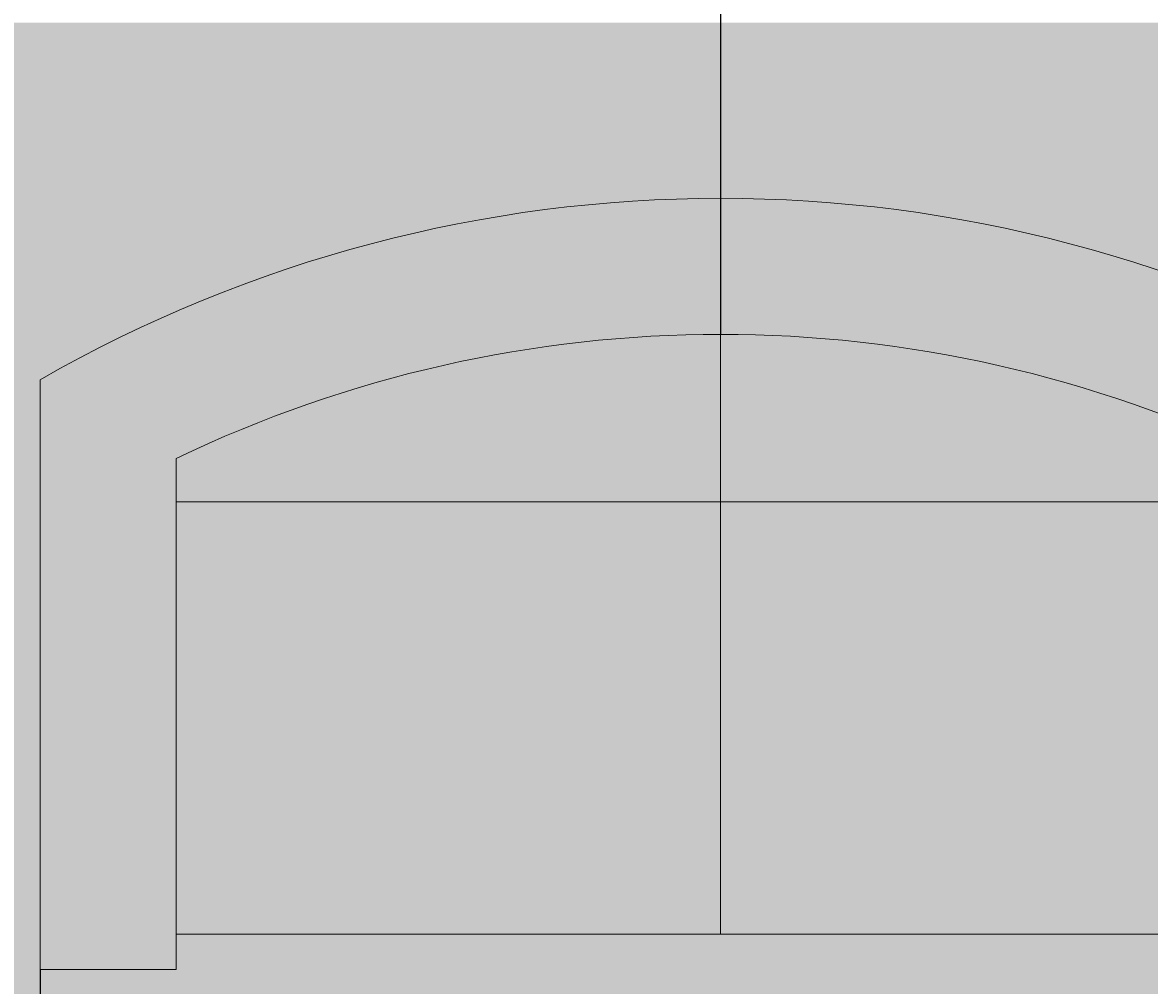
# Model space of a CAD drawing. Units: millimetres. Extents: x -229 to 16545, y -10488 to 4272.
# Tile 21 of 29: x 11572 to 12629, y -2111 to -1208. Entities that reach past the tile are written whole.
import ezdxf

# ---------------------------------------------------------------- set-up
doc = ezdxf.new("R2010")
doc.units = ezdxf.units.MM
for name, color, linetype, lineweight in [('A-ANNO-DIMS', 2, 'Continuous', 18), ('A-FURN', 8, 'Continuous', 18), ('A-FURN-PATT', 252, 'Continuous', 13)]:
    doc.layers.add(name, color=color, linetype=linetype, lineweight=lineweight)
doc.layers.add('A-FLOR-PATT', color=254, linetype='Continuous', lineweight=13, true_color=0xfeeab9)
doc.styles.get("Standard").update_dxf_attribs({"font": 'arial.ttf'})
doc.dimstyles.get("Standard").update_dxf_attribs({"dimtxt": 0.18, "dimasz": 0.18, "dimexe": 0.18, "dimexo": 0.0625, "dimgap": 0.09, "dimtad": 0, "dimtih": 1, "dimtoh": 1, "dimdec": 4, "dimzin": 0, "dimdsep": 46, "dimtxsty": 'Standard', "dimcen": 0.09, "dimadec": 0, "dimazin": 0, "dimtfac": 1, "dimtdec": 4, "dimtofl": 0, "dimtmove": 0, "dimatfit": 3, "dimfxl": 1, "dimtolj": 1, "dimtzin": 0, "dimarcsym": 0})

# ---------------------------------------------------------------- blocks, each defined once
blk = doc.blocks.new('Sofa - Roundback Loveseat 5 ft.')
for p, q in [((0, -32.44198), (0, -5.99998)), ((-24, -33.99998), (-24, -11.46958)), ((-23.9998, -13.38178), (23.99986, -13.38178)), ((-24, -32.44198), (24.00004, -32.44198))]:
    blk.add_line(p, q)
blk.add_lwpolyline([(-24, -33.99998), (-30, -33.99998), (-30, -7.99998)])
for centre, radius, start, end in [((0, -60.24998), 60.24998, 60.13715, 119.8628), ((0, -61.38438), 55.38444, 64.32083, 115.6792)]:
    blk.add_arc(centre, radius, start, end)
blk = doc.blocks.new('*D39')
at = {"layer": 'A-ANNO-DIMS', "color": 0, "lineweight": -2, "transparency": 16777216}
for p, q in [((11588.8, -2096.3), (11588.8, -2287.9)), ((12864.9, -2096.3), (12864.9, -2287.9)), ((11588.9, -2287.7), (12225.8, -2287.7)), ((12864.7, -2287.7), (12227.9, -2287.7))]:
    blk.add_line(p, q, dxfattribs=at)
at = {"layer": 'A-ANNO-DIMS', "color": 0, "transparency": 16777216}
for points in [[(11588.9, -2287.7), (11588.9, -2287.7), (11588.8, -2287.7)], [(12864.7, -2287.7), (12864.7, -2287.7), (12864.9, -2287.7)]]:
    blk.add_solid(points, dxfattribs=at)
at = {"layer": 'Defpoints', "color": 0, "transparency": 16777216}
for p in [(11588.8, -2096.3), (12864.9, -2096.3), (12864.9, -2287.7)]:
    blk.add_point(p, dxfattribs=at)
at = {"layer": 'A-ANNO-DIMS', "color": 0, "transparency": 16777216, "insert": (12226.8, -2287.7), "char_height": 0.18, "attachment_point": 5}
blk.add_mtext('\\A1;LOVESEAT 1276', dxfattribs=at)
blk = doc.blocks.new('*D103')
at = {"layer": 'A-ANNO-DIMS', "color": 0, "lineweight": -2, "transparency": 16777216}
for p, q in [((12227, -604.2), (12226.8, -604.2)), ((12226.8, -604.2), (12226.8, -1372.9)), ((12226.7, -2654.6), (12226.9, -2654.6)), ((12226.8, -2654.7), (12226.8, -2654.5))]:
    blk.add_line(p, q, dxfattribs=at)
at = {"layer": 'A-ANNO-DIMS', "color": 0, "transparency": 16777216}
blk.add_solid([(12226.8, -1372.9), (12226.9, -1372.9), (12226.8, -1373.1)], dxfattribs=at)
at = {"layer": 'Defpoints', "color": 0, "transparency": 16777216}
for p in [(12226.8, -1373.1), (12226.8, -2654.6)]:
    blk.add_point(p, dxfattribs=at)
at = {"layer": 'A-ANNO-DIMS', "color": 0, "transparency": 16777216, "insert": (12227.6, -604.2), "char_height": 0.18, "attachment_point": 5}
blk.add_mtext('\\A1;R1281.5', dxfattribs=at)
blk = doc.blocks.new('*D104')
at = {"layer": 'A-ANNO-DIMS', "color": 0, "lineweight": -2, "transparency": 16777216}
for p, q in [((12227, -793.9), (12226.8, -793.9)), ((12226.8, -793.9), (12226.8, -1500.5)), ((12226.7, -2678.7), (12226.9, -2678.7)), ((12226.8, -2678.8), (12226.8, -2678.6))]:
    blk.add_line(p, q, dxfattribs=at)
at = {"layer": 'A-ANNO-DIMS', "color": 0, "transparency": 16777216}
blk.add_solid([(12226.8, -1500.5), (12226.9, -1500.5), (12226.8, -1500.7)], dxfattribs=at)
at = {"layer": 'Defpoints', "color": 0, "transparency": 16777216}
for p in [(12226.8, -1500.7), (12226.8, -2678.7)]:
    blk.add_point(p, dxfattribs=at)
at = {"layer": 'A-ANNO-DIMS', "color": 0, "transparency": 16777216, "insert": (12227.5, -793.9), "char_height": 0.18, "attachment_point": 5}
blk.add_mtext('\\A1;R1178', dxfattribs=at)

msp = doc.modelspace()

# ---------------------------------------------------------------- hatches: boundary and pattern name
at = {"layer": 'A-FLOR-PATT', "transparency": 33554592}
h = msp.add_hatch(color=256, dxfattribs=at)
h.dxf.hatch_style = 1
h.paths.add_polyline_path([(7975.933, -5325.772), (7943.121, -5325.772), (7943.121, -4576.49, 0.40145271), (7225.933, -5325.772, 0.40145271), (6508.746, -4576.49), (6508.746, -5325.772), (6475.933, -5325.772), (6475.933, -5438.272), (5975.933, -5438.272), (5975.933, -7267.724), (5975.933, -7438.272), (6478.619, -7438.272), (6463.448, -7355.919), (6464.88, -7356.837), (6463.849, -7358.097), (6478.619, -7438.272), (6610.327, -7438.272), (6632.656, -7409.564), (6632.525, -7406.967), (6634.208, -7407.569), (6619.273, -7426.77), (6654.466, -7438.272), (7610.517, -7438.272), (7607.41, -7421.409), (7608.842, -7422.327), (7607.812, -7423.587), (7610.517, -7438.272), (7975.933, -7438.272)])
h.paths.add_polyline_path([(13785.933, -1208.272), (9555.933, -1208.272), (9555.933, -961.785), (9705.933, -961.785), (9705.933, -918.035), (10704.976, -918.035, 0.40145271), (9705.933, 38.215), (9555.933, 38.215), (9555.933, 2021.728), (5975.933, 2021.728), (5975.933, 755.492), (5745.933, 755.492), (5745.933, 1427.266), (2918.813, 1427.266), (2918.813, -492.942), (5013.319, -492.942), (5013.319, -978.272), (5745.933, -978.272), (5745.933, -397.513), (5975.933, -397.513), (5975.933, -1208.272), (4560.933, -1208.272), (4560.933, -1265.772), (4448.433, -1265.772), (4448.433, -1298.585), (4445.933, -1298.585), (3699.151, -1298.585, 0.40145271), (4448.433, -2015.772), (4560.933, -2015.772), (4560.933, -2384.177), (5745.933, -2384.177), (5799.402, -2384.177), (5799.402, -4518.272), (5975.933, -4518.272), (5975.933, -5208.272), (6475.933, -5208.272), (6475.933, -4575.772), (6508.746, -4575.772), (6508.746, -4576.49, -0.35647263), (7216.672, -5208.272), (7235.194, -5208.272, -0.35647263), (7943.121, -4576.49), (7943.121, -4575.772), (7975.933, -4575.772), (7975.933, -5208.272), (11176.247, -5208.272), (11159.44, -5191.465), (10520.768, -5191.465), (10520.768, -4888.936), (10571.19, -4888.936), (10571.19, -4872.129), (10772.876, -4872.129), (10772.876, -4888.936), (10789.683, -4888.936), (10789.683, -4872.129), (10991.368, -4872.129), (10991.368, -4888.936), (11041.79, -4888.936), (11041.79, -4872.129), (11058.597, -4872.129, -0.09090909), (11428.354, -4872.129), (11445.162, -4872.129), (11445.162, -4888.936), (11529.197, -4888.936), (11529.197, -5191.465), (11327.512, -5191.465), (11310.704, -5208.272), (13785.933, -5208.272)])
h.paths.add_polyline_path([(11047.216, -1630.944, -1), (11402.816, -1630.944, -1)], flags=16)
h.paths.add_polyline_path([(11148.816, -1630.944), (11225.016, -1554.744), (11301.216, -1630.944), (11225.016, -1707.144)], flags=0)
h.paths.add_polyline_path([(11199.616, -1630.944, -1), (11250.416, -1630.944, -1)], flags=0)
h.paths.add_polyline_path([(11588.751, -2096.259), (11588.751, -1543.254, -0.26666697), (12864.918, -1543.254), (12864.918, -2096.259), (12737.302, -2096.259), (12737.302, -2063.121), (11716.368, -2063.121), (11716.368, -2096.259)], flags=16)
h.paths.add_polyline_path([(12012.696, -2489.42), (12600.997, -2489.42), (12600.997, -3666.022), (12012.696, -3666.022)], flags=16)
h.paths.add_polyline_path([(12176.41, -3599.403), (12174.938, -3609.076), (12173.789, -3618.819), (12173.09, -3628.559), (12172.973, -3638.221), (12173.89, -3652.852), (12175.008, -3657.025), (12172.909, -3643.473), (12173.142, -3624.297), (12175.386, -3605.273)], flags=0)
h.paths.add_polyline_path([(8026.289, -286.944), (7737.703, -287.19), (7734.87, -269.156), (8029.092, -268.905)], flags=16)
h.paths.add_polyline_path([(7733.453, -260.139), (7710.784, -115.865), (7557.191, -115.996), (7556.999, 109.744), (7412.687, 132.166), (7412.433, 429.206), (7556.707, 451.876), (7556.568, 614.769), (7412.256, 637.19), (7412.003, 934.231), (7556.276, 956.9), (7556.084, 1182.639), (7709.677, 1182.77), (7732.099, 1327.082), (8029.14, 1327.335), (8051.808, 1183.062), (8205.401, 1183.192), (8205.594, 957.454), (8349.906, 935.031), (8350.159, 637.99), (8205.885, 615.322), (8206.024, 452.43), (8350.336, 430.006), (8350.59, 132.965), (8206.316, 110.298), (8206.509, -115.442), (8052.916, -115.573), (8030.493, -259.885)], flags=16)
h.paths.add_polyline_path([(12261.416, -3475.554), (12262.632, -3486.776), (12264.032, -3497.007), (12265.554, -3506.365), (12267.136, -3514.968), (12268.719, -3522.935), (12271.304, -3535.59), (12273.606, -3548.078), (12275.271, -3561.064), (12275.93, -3574.938), (12275.325, -3590.3), (12273.425, -3607.964), (12270.795, -3625.658), (12268.066, -3641.063), (12266.318, -3649.679), (12265.456, -3653.626), (12263.984, -3659.846), (12264.032, -3659.566), (12264.342, -3658.241), (12264.807, -3656.37), (12265.456, -3653.626), (12266.318, -3649.679), (12267.409, -3644.302), (12268.668, -3637.664), (12270.019, -3630.037), (12271.384, -3621.695), (12272.69, -3612.908), (12273.857, -3603.948), (12274.81, -3595.088), (12275.47, -3586.601), (12275.782, -3578.689), (12275.757, -3571.292), (12275.423, -3564.275), (12274.816, -3557.512), (12273.964, -3550.872), (12272.896, -3544.224), (12271.645, -3537.439), (12270.24, -3530.385), (12267.543, -3517.181), (12264.612, -3501.247), (12261.849, -3481.059)], flags=0)
h.paths.add_polyline_path([(12332.136, -3408.03), (12333.483, -3416.79), (12335.077, -3424.54), (12336.915, -3431.355), (12338.991, -3437.32), (12341.266, -3442.55), (12343.694, -3447.166), (12346.229, -3451.292), (12348.826, -3455.051), (12351.438, -3458.563), (12357.476, -3466.491), (12363.61, -3476.575), (12368.309, -3489.762), (12369.929, -3503.427), (12369.842, -3516.511), (12368.43, -3530.867), (12365.816, -3545.835), (12362.382, -3559.786), (12360.968, -3564.487), (12363.063, -3557.021), (12364.898, -3549.566), (12366.473, -3542.077), (12367.773, -3534.631), (12368.781, -3527.301), (12369.483, -3520.162), (12369.863, -3513.291), (12369.906, -3506.759), (12369.599, -3500.643), (12368.93, -3494.999), (12367.924, -3489.796), (12366.61, -3484.994), (12365.024, -3480.542), (12363.19, -3476.399), (12361.141, -3472.516), (12358.909, -3468.847), (12356.525, -3465.347), (12354.02, -3461.954), (12351.438, -3458.563), (12345.462, -3450.529), (12339.923, -3439.996), (12335.85, -3428.296), (12332.68, -3412.888)], flags=0)
h.paths.add_polyline_path([(12385.287, -3334.612), (12384.977, -3342.409), (12385.02, -3349.196), (12385.4, -3355.066), (12386.104, -3360.105), (12387.112, -3364.41), (12388.412, -3368.071), (12389.987, -3371.181), (12391.823, -3373.832), (12393.919, -3376.097), (12396.337, -3377.978), (12399.153, -3379.462), (12402.445, -3380.531), (12406.289, -3381.172), (12410.758, -3381.371), (12415.935, -3381.106), (12421.893, -3380.368), (12428.658, -3379.159), (12436.069, -3377.55), (12443.907, -3375.635), (12451.961, -3373.505), (12460.015, -3371.254), (12467.853, -3368.971), (12475.263, -3366.749), (12482.029, -3364.68), (12491.877, -3361.657), (12497.701, -3360.107), (12501.639, -3359.288), (12510.135, -3358.326), (12519.662, -3365.412), (12524.243, -3378.911), (12523.764, -3390.7), (12520.746, -3401.577), (12514.248, -3415.634), (12511.518, -3420.418), (12515.856, -3412.154), (12519.153, -3405.024), (12521.516, -3398.804), (12523.049, -3393.276), (12523.865, -3388.212), (12524.059, -3383.441), (12523.7, -3378.958), (12522.853, -3374.815), (12521.576, -3371.054), (12519.931, -3367.722), (12517.982, -3364.865), (12515.786, -3362.529), (12513.405, -3360.758), (12510.877, -3359.588), (12508.136, -3358.982), (12505.086, -3358.897), (12501.639, -3359.288), (12497.701, -3360.107), (12493.183, -3361.309), (12487.988, -3362.851), (12476.403, -3366.408), (12463.335, -3370.326), (12447.372, -3374.788), (12431.759, -3378.604), (12418.504, -3380.974), (12405.811, -3381.624), (12394.725, -3378.025), (12388.039, -3368.367), (12385.583, -3357.877), (12384.826, -3346.204), (12385.428, -3331.059), (12385.953, -3325.719)], flags=0)
h.paths.add_polyline_path([(7880.016, 1173.969), (7880.373, 1175.495), (7880.433, 1175.851), (7879.484, 1171.818)], flags=0)
h.paths.add_polyline_path([(7802.33, 874.962), (7800.771, 885.032), (7798.932, 893.941), (7796.811, 901.774), (7794.419, 908.63), (7791.798, 914.639), (7789.002, 919.945), (7786.083, 924.686), (7783.093, 929.005), (7780.087, 933.043), (7774.996, 939.717), (7768.406, 949.37), (7762.174, 963.427), (7759.342, 978.002), (7758.629, 991.888), (7759.492, 1007.928), (7761.801, 1025.496), (7765.392, 1044.035), (7766.625, 1049.048), (7764.522, 1039.543), (7762.719, 1030.232), (7761.232, 1021.168), (7760.08, 1012.405), (7759.28, 1003.994), (7758.849, 995.988), (7758.806, 988.44), (7759.167, 981.404), (7759.942, 974.914), (7761.104, 968.936), (7762.617, 963.414), (7764.448, 958.299), (7766.559, 953.535), (7768.918, 949.073), (7771.487, 944.856), (7774.232, 940.835), (7777.115, 936.938), (7782.377, 930.041), (7787.845, 922.139), (7793.348, 911.698), (7798.042, 898.247), (7801.702, 880.527)], flags=0)
h.paths.add_polyline_path([(12519.068, -3228.534), (12519.615, -3236.235), (12520.529, -3242.343), (12521.78, -3247.103), (12523.337, -3250.758), (12525.171, -3253.556), (12527.248, -3255.709), (12529.522, -3257.296), (12531.95, -3258.361), (12534.486, -3258.949), (12537.082, -3259.11), (12539.694, -3258.888), (12542.277, -3258.329), (12544.781, -3257.478), (12547.173, -3256.388), (12549.46, -3255.129), (12550.455, -3254.517), (12555.825, -3251.109), (12557.835, -3249.942), (12565.181, -3246.404), (12574.565, -3253.032), (12576.931, -3265.022), (12576.627, -3277.425), (12575.416, -3290.819), (12574.851, -3295.392), (12575.708, -3287.593), (12576.322, -3280.806), (12576.688, -3274.939), (12576.812, -3269.899), (12576.688, -3265.593), (12576.322, -3261.932), (12575.708, -3258.822), (12574.851, -3256.172), (12573.753, -3253.905), (12572.439, -3252.005), (12570.943, -3250.474), (12569.293, -3249.309), (12567.523, -3248.513), (12565.658, -3248.083), (12563.732, -3248.022), (12561.777, -3248.328), (12559.814, -3248.989), (12557.835, -3249.942), (12555.825, -3251.109), (12553.77, -3252.413), (12551.652, -3253.78), (12549.46, -3255.129), (12543.167, -3258.594), (12532.661, -3259.485), (12524.685, -3253.923), (12520.949, -3245.152), (12519.138, -3233.042)], flags=0)
h.paths.add_polyline_path([(7741.293, 790.501), (7741.641, 799.467), (7741.584, 807.269), (7741.141, 814.015), (7740.329, 819.809), (7739.165, 824.757), (7737.667, 828.966), (7735.853, 832.541), (7733.74, 835.586), (7731.348, 838.188), (7728.71, 840.348), (7725.861, 842.052), (7722.836, 843.28), (7719.671, 844.015), (7716.4, 844.237), (7713.06, 843.932), (7709.684, 843.081), (7706.304, 841.686), (7702.923, 839.834), (7699.543, 837.629), (7696.164, 835.178), (7692.784, 832.585), (7684.718, 826.315), (7675.609, 820.63), (7664.001, 817.274), (7654.105, 821.884), (7647.171, 832.02), (7644.191, 846.522), (7646.321, 860.288), (7647.49, 864.223), (7645.946, 857.865), (7645.046, 852.044), (7644.827, 846.557), (7645.243, 841.404), (7646.221, 836.642), (7647.693, 832.318), (7649.587, 828.489), (7651.832, 825.206), (7654.359, 822.523), (7657.097, 820.49), (7659.984, 819.145), (7662.993, 818.452), (7666.108, 818.357), (7669.311, 818.809), (7672.583, 819.755), (7675.908, 821.139), (7679.268, 822.913), (7682.645, 825.021), (7686.025, 827.401), (7689.404, 829.958), (7692.784, 832.585), (7700.505, 838.509), (7709.871, 843.64), (7721.436, 844.698), (7733.277, 837.617), (7739.571, 825.214), (7741.557, 811.049), (7741.669, 795.575)], flags=0)
h.paths.add_polyline_path([(8377.641, 137.216), (8359.607, 134.382), (8359.356, 428.605), (8377.395, 425.802)], flags=16)
h.paths.add_polyline_path([(7650.715, 668.465), (7650.08, 677.319), (7649.023, 684.34), (7647.579, 689.811), (7645.785, 694.012), (7643.675, 697.228), (7641.286, 699.7), (7638.669, 701.521), (7635.876, 702.744), (7632.96, 703.419), (7629.974, 703.601), (7626.971, 703.344), (7624.004, 702.697), (7621.125, 701.717), (7618.375, 700.462), (7615.749, 699.013), (7614.561, 698.279), (7608.435, 694.382), (7606.125, 693.04), (7598.981, 689.594), (7589.669, 693.773), (7585.26, 702.856), (7584.221, 713.11), (7584.49, 724.584), (7585.863, 739.937), (7586.518, 745.277), (7585.539, 736.31), (7584.841, 728.507), (7584.424, 721.761), (7584.288, 715.966), (7584.433, 711.016), (7584.86, 706.807), (7585.567, 703.231), (7586.556, 700.186), (7587.821, 697.58), (7589.332, 695.397), (7591.053, 693.637), (7592.951, 692.3), (7594.989, 691.385), (7597.132, 690.895), (7599.346, 690.826), (7601.594, 691.18), (7603.851, 691.943), (7606.125, 693.04), (7608.435, 694.382), (7610.797, 695.885), (7613.229, 697.458), (7620.475, 701.929), (7632.001, 704.44), (7643.476, 699.417), (7648.536, 687.571), (7650.63, 673.661)], flags=0)
h.paths.add_polyline_path([(7385.628, 136.37), (7385.382, 424.956), (7403.416, 427.789), (7403.667, 133.567)], flags=16)
h.paths.add_polyline_path([(12993.884, -2257.186), (12959.588, -2257.186), (12959.588, -2125.099), (13531.966, -2125.099, -0.19047621), (13531.966, -3974.321), (12959.588, -3974.321), (12959.588, -3842.233), (12993.884, -3842.233)], flags=16)
h.paths.add_polyline_path([(13413.486, -3313.884), (13413.486, -2785.535), (13562.885, -2785.535, -0.04962821), (13562.885, -3313.884)], flags=0)
h.paths.add_polyline_path([(8377.21, 642.241), (8359.176, 639.407), (8358.925, 933.629), (8376.964, 930.826)], flags=16)
h.paths.add_polyline_path([(13086.058, -1864.83), (13086.058, -1449.84), (13501.048, -1449.84), (13501.048, -1864.83)], flags=16)
h.paths.add_polyline_path([(13305.814, -1862.197), (13302.103, -1859.624), (13298.088, -1857.068), (13293.799, -1854.536), (13289.262, -1852.031), (13284.504, -1849.559), (13279.554, -1847.125), (13274.439, -1844.735), (13269.17, -1842.389), (13263.701, -1840.081), (13257.97, -1837.797), (13251.914, -1835.525), (13245.472, -1833.252), (13238.582, -1830.968), (13231.18, -1828.66), (13223.206, -1826.315), (13209.182, -1822.458), (13204.584, -1821.48), (13217.962, -1824.773), (13235.072, -1829.804), (13248.777, -1834.349), (13260.829, -1838.869), (13274.479, -1844.63), (13289.675, -1852.101), (13302.553, -1859.704)], flags=0)
h.paths.add_polyline_path([(13428.104, -1820.994), (13419.007, -1818.141), (13409.95, -1815.4), (13400.766, -1812.747), (13391.271, -1810.151), (13376.087, -1806.251), (13370.618, -1805.019), (13386.304, -1808.794), (13405.087, -1813.928), (13423.014, -1819.354)], flags=0)
h.paths.add_polyline_path([(7385.197, 641.395), (7384.951, 929.98), (7402.986, 932.814), (7403.236, 638.592)], flags=16)
h.paths.add_polyline_path([(13262.537, -1725.526), (13253.246, -1724.74), (13244.516, -1724.117), (13235.94, -1723.625), (13223.267, -1723.062), (13217.598, -1722.912), (13231.966, -1723.397), (13248.733, -1724.359), (13266.899, -1725.895), (13272.802, -1726.502)], flags=0)
h.paths.add_polyline_path([(13191.893, -1641.137), (13208.675, -1640.506), (13214.057, -1640.258), (13197.763, -1640.936)], flags=0)
h.paths.add_polyline_path([(13097.524, -1608.457), (13114.284, -1609.031), (13120.126, -1609.105), (13103.045, -1608.71)], flags=0)
h.paths.add_polyline_path([(13465.328, -1521.577), (13473.906, -1517.015), (13481.761, -1511.636), (13492.562, -1502.076), (13495.327, -1497.933), (13485.818, -1508.858), (13470.208, -1519.547)], flags=0)
h.paths.add_polyline_path([(13175.015, -1500.891), (13184.046, -1501.807), (13192.721, -1502.52), (13201.114, -1503.034), (13209.273, -1503.351), (13217.244, -1503.476), (13225.078, -1503.41), (13232.821, -1503.16), (13240.524, -1502.728), (13248.233, -1502.117), (13255.993, -1501.322), (13263.825, -1500.293), (13271.746, -1498.974), (13279.775, -1497.305), (13287.928, -1495.229), (13296.222, -1492.688), (13304.675, -1489.622), (13313.304, -1485.975), (13322.089, -1481.727), (13330.859, -1477.028), (13339.408, -1472.063), (13347.526, -1467.02), (13355.006, -1462.087), (13364.86, -1455.202), (13367.224, -1453.299), (13358.544, -1459.754), (13343.348, -1469.775), (13326.143, -1479.767), (13309.023, -1488.045), (13292.249, -1494.129), (13276.009, -1498.264), (13260.299, -1500.88), (13244.401, -1502.51), (13228.945, -1503.378), (13213.316, -1503.508), (13197.047, -1502.876), (13180.088, -1501.481)], flags=0)
h.paths.add_polyline_path([(7733.501, 1336.101), (7736.303, 1354.14), (8024.889, 1354.386), (8027.723, 1336.352)], flags=16)
at = {"layer": 'A-FURN-PATT'}
h = msp.add_hatch(color=256, dxfattribs=at)
h.dxf.hatch_style = 1
h.paths.add_polyline_path([(13413.486, -2257.186), (12993.884, -2257.186), (12993.884, -2785.535), (13413.486, -2785.535)], flags=17)
h.paths.add_polyline_path([(13413.486, -2785.535), (12993.884, -2785.535), (12993.884, -3313.884), (13413.486, -3313.884)], flags=17)
h.paths.add_polyline_path([(13413.486, -3313.884), (12993.884, -3313.884), (12993.884, -3842.233), (13413.486, -3842.233)], flags=17)
h.paths.add_polyline_path([(13531.966, -2125.099), (12959.588, -2125.099), (12959.588, -2257.186), (13455.573, -2257.186, -0.15194781), (13455.573, -3842.233), (12959.588, -3842.233), (12959.588, -3974.321), (13531.966, -3974.321, 0.19047621)])
h.paths.add_polyline_path([(13455.573, -2257.186), (13413.486, -2257.186), (13413.486, -2785.535), (13562.885, -2785.535, 0.05064665)], flags=17)
h.paths.add_polyline_path([(13562.885, -2785.535), (13413.486, -2785.535), (13413.486, -3313.884), (13562.885, -3313.884, 0.04962821)], flags=17)
h.paths.add_polyline_path([(13562.885, -3313.884), (13413.486, -3313.884), (13413.486, -3842.233), (13455.573, -3842.233, 0.05064665)], flags=17)
h.paths.add_polyline_path([(11588.751, -1543.254), (11588.751, -2096.259), (11716.368, -2096.259), (11716.368, -1617.061, -0.22792319), (12737.302, -1617.061), (12737.302, -2096.259), (12864.918, -2096.259), (12864.918, -1543.254, 0.26666697)])
h.paths.add_polyline_path([(12226.834, -1500.713, 0.11251869), (11716.368, -1617.061), (11716.368, -1657.721), (12226.834, -1657.721)], flags=17)
h.paths.add_polyline_path([(12737.302, -1617.061, 0.11251889), (12226.834, -1500.713), (12226.834, -1657.721), (12737.302, -1657.721)], flags=17)
h.paths.add_polyline_path([(12226.834, -1657.721), (11716.368, -1657.721), (11716.368, -2063.121), (12226.834, -2063.121)], flags=17)
h.paths.add_polyline_path([(12737.302, -1657.721), (12226.834, -1657.721), (12226.834, -2063.121), (12737.302, -2063.121)], flags=17)

# ---------------------------------------------------------------- block references
at = {"layer": 'A-FURN', "xscale": 21.26944187666239, "yscale": 21.26944187666239, "zscale": 21.26944187666239}
msp.add_blockref('Sofa - Roundback Loveseat 5 ft.', (12226.834, -1373.098), dxfattribs=at)

# ---------------------------------------------------------------- dimensions: what is measured, and where the dimension line sits
at = {"layer": 'A-ANNO-DIMS'}
for center, mpoint, override, picture, middle in [((12226.834, -2654.582), (12226.835, -1373.098), {"dimdec": 1, "dimlfac": 1, "dimrnd": 0, "dimzin": 0, "dimdsep": 46, "dimlunit": 2}, '*D103', (12227.565, -604.208)), ((12226.834, -2678.71), (12226.834, -1500.713), {"dimdec": 0, "dimlfac": 1, "dimrnd": 0, "dimzin": 0, "dimdsep": 46, "dimlunit": 2}, '*D104', (12227.459, -793.916))]:
    dim = msp.add_radius_dim(center=center, mpoint=mpoint, dimstyle='Standard', override=override, dxfattribs=at)
    dim.commit()
    dim.dimension.update_dxf_attribs({"geometry": picture, "text_midpoint": middle, "dimtype": 164})
dim = msp.add_linear_dim(base=(12864.918, -2287.684), p1=(11588.751, -2096.259), p2=(12864.918, -2096.259), text='LOVESEAT <>', dimstyle='Standard', override={"dimdec": 0, "dimlfac": 1, "dimrnd": 0, "dimzin": 0, "dimdsep": 46, "dimlunit": 2}, dxfattribs=at)
dim.commit()
dim.dimension.update_dxf_attribs({"geometry": '*D39', "text_midpoint": (12226.835, -2287.684)})

doc.saveas('drawing.dxf')
